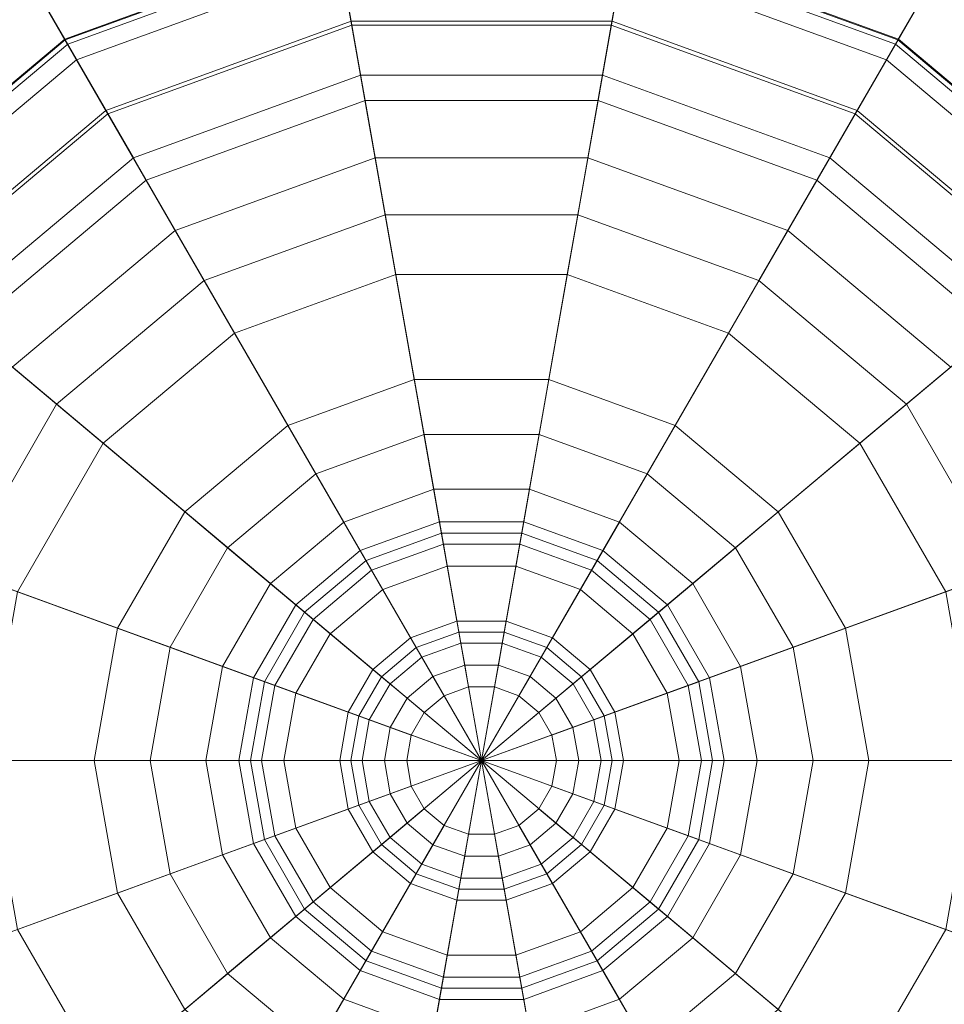
# Model space of a CAD drawing. Units: inches. Extents: x 375 to 1122, y 27 to 1069.
# Tile 141 of 155: x 732.384 to 733.741, y 898.759 to 900.205. Entities that reach past the tile are written whole.
import ezdxf

# ---------------------------------------------------------------- set-up
doc = ezdxf.new("R2010")
doc.units = ezdxf.units.IN
doc.layers.add('A-ANNO-DIMS', color=2, linetype='Continuous', lineweight=18)
doc.layers.add('Furniture', color=30, linetype='Continuous', lineweight=18)
doc.styles.get("Standard").update_dxf_attribs({"font": 'arial.ttf'})
doc.dimstyles.new('ISO-25', dxfattribs={"dimtxt": 12, "dimasz": 2.5, "dimexe": 1.5, "dimexo": 1.5, "dimtad": 1, "dimdec": 1, "dimlunit": 3, "dimtxsty": 'Standard', "dimblk": 'ARCHTICK', "dimcen": 2.5, "dimadec": 0, "dimazin": 0, "dimtfac": 1, "dimtdec": 1, "dimtmove": 0, "dimatfit": 3, "dimfxl": 1.5, "dimfxlon": 1, "dimarcsym": 0})

# ---------------------------------------------------------------- blocks, each defined once
blk = doc.blocks.new('A$C403C54AD')
for points in [[(0.980157, 1.23678, -0.04658), (0.980157, 1.202917, -0.043501), (0.980157, 1.202917, -0.043501), (0.968576, 1.234737, -0.04658)], [(0.991739, 1.234737, -0.04658), (0.980157, 1.202917, -0.043501), (0.980157, 1.202917, -0.043501), (0.980157, 1.23678, -0.04658)], [(0.968576, 1.234737, -0.04658), (0.980157, 1.202917, -0.043501), (0.980157, 1.202917, -0.043501), (0.958391, 1.228857, -0.04658)], [(1.001923, 1.228857, -0.04658), (0.980157, 1.202917, -0.043501), (0.980157, 1.202917, -0.043501), (0.991739, 1.234737, -0.04658)], [(0.980157, 1.217132, -0.040074), (0.980157, 1.233514, -0.043349), (0.969693, 1.231669, -0.043349), (0.975296, 1.216274, -0.040074)], [(0.985019, 1.216274, -0.040074), (0.990622, 1.231669, -0.043349), (0.980157, 1.233514, -0.043349), (0.980157, 1.217132, -0.040074)], [(0.975296, 1.216274, -0.040074), (0.969693, 1.231669, -0.043349), (0.96049, 1.226356, -0.043349), (0.971021, 1.213806, -0.040074)], [(0.989294, 1.213806, -0.040074), (0.999824, 1.226356, -0.043349), (0.990622, 1.231669, -0.043349), (0.985019, 1.216274, -0.040074)], [(0.958391, 1.228857, -0.04658), (0.980157, 1.202917, -0.043501), (0.980157, 1.202917, -0.043501), (0.950832, 1.219849, -0.04658)], [(0.96049, 1.226356, -0.043349), (0.958391, 1.228857, -0.04658), (0.950832, 1.219849, -0.04658), (0.95366, 1.218216, -0.043349)], [(0.960516, 1.226325, 0.116404), (0.958647, 1.228552, 0.10318), (0.951177, 1.219649, 0.10318), (0.953695, 1.218195, 0.116404)], [(0.958647, 1.228552, 0.10318), (0.959081, 1.228035, 0.074938), (0.951762, 1.219312, 0.074938), (0.951177, 1.219649, 0.10318)], [(0.970778, 1.228687, 0.056929), (0.973195, 1.222047, 0.046697), (0.967072, 1.218512, 0.046697), (0.96253, 1.223925, 0.056929)], [(1.009483, 1.219849, -0.04658), (0.980157, 1.202917, -0.043501), (0.980157, 1.202917, -0.043501), (1.001923, 1.228857, -0.04658)], [(0.997785, 1.223925, 0.056929), (0.993243, 1.218512, 0.046697), (0.98712, 1.222047, 0.046697), (0.989537, 1.228687, 0.056929)], [(0.959081, 1.228035, 0.074938), (0.96253, 1.223925, 0.056929), (0.956408, 1.216629, 0.056929), (0.951762, 1.219312, 0.074938)], [(0.971021, 1.213806, -0.040074), (0.96049, 1.226356, -0.043349), (0.95366, 1.218216, -0.043349), (0.967847, 1.210025, -0.040074)], [(0.963728, 1.222497, 0.12581), (0.960516, 1.226325, 0.116404), (0.953695, 1.218195, 0.116404), (0.958022, 1.215697, 0.12581)], [(0.96063, 1.226189, 0.102963), (0.962436, 1.224037, 0.115599), (0.956282, 1.216702, 0.115599), (0.953848, 1.218107, 0.102963)], [(0.961053, 1.225685, 0.075423), (0.96063, 1.226189, 0.102963), (0.953848, 1.218107, 0.102963), (0.954418, 1.217778, 0.075423)], [(0.973957, 1.219951, 0.048884), (0.971739, 1.226046, 0.058276), (0.964336, 1.221772, 0.058276), (0.968505, 1.216804, 0.048884)], [(0.991809, 1.216804, 0.048884), (0.995978, 1.221772, 0.058276), (0.988575, 1.226046, 0.058276), (0.986357, 1.219951, 0.048884)], [(0.964336, 1.221772, 0.058276), (0.961053, 1.225685, 0.075423), (0.954418, 1.217778, 0.075423), (0.958842, 1.215224, 0.058276)], [(0.962436, 1.224037, 0.115599), (0.965707, 1.220139, 0.12581), (0.960688, 1.214158, 0.12581), (0.956282, 1.216702, 0.115599)], [(0.96253, 1.223925, 0.056929), (0.967072, 1.218512, 0.046697), (0.962527, 1.213096, 0.046697), (0.956408, 1.216629, 0.056929)], [(0.980157, 1.223275, 0.046697), (0.980157, 1.213036, 0.03933), (0.976696, 1.212426, 0.03933), (0.973195, 1.222047, 0.046697)], [(0.98712, 1.222047, 0.046697), (0.983618, 1.212426, 0.03933), (0.980157, 1.213036, 0.03933), (0.980157, 1.223275, 0.046697)], [(0.965707, 1.220139, 0.12581), (0.963728, 1.222497, 0.12581), (0.958022, 1.215697, 0.12581), (0.960688, 1.214158, 0.12581)], [(0.973195, 1.222047, 0.046697), (0.976696, 1.212426, 0.03933), (0.973653, 1.210669, 0.03933), (0.967072, 1.218512, 0.046697)], [(0.993243, 1.218512, 0.046697), (0.986661, 1.210669, 0.03933), (0.983618, 1.212426, 0.03933), (0.98712, 1.222047, 0.046697)], [(0.968505, 1.216804, 0.048884), (0.964336, 1.221772, 0.058276), (0.958842, 1.215224, 0.058276), (0.964459, 1.211981, 0.048884)], [(0.980157, 1.211822, 0.042248), (0.980157, 1.221045, 0.048884), (0.973957, 1.219951, 0.048884), (0.977112, 1.211285, 0.042248)], [(0.983203, 1.211285, 0.042248), (0.986357, 1.219951, 0.048884), (0.980157, 1.221045, 0.048884), (0.980157, 1.211822, 0.042248)], [(0.977112, 1.211285, 0.042248), (0.973957, 1.219951, 0.048884), (0.968505, 1.216804, 0.048884), (0.974434, 1.209738, 0.042248)], [(0.985881, 1.209738, 0.042248), (0.991809, 1.216804, 0.048884), (0.986357, 1.219951, 0.048884), (0.983203, 1.211285, 0.042248)], [(0.950832, 1.219849, -0.04658), (0.980157, 1.202917, -0.043501), (0.980157, 1.202917, -0.043501), (0.94681, 1.208798, -0.04658)], [(0.95366, 1.218216, -0.043349), (0.950832, 1.219849, -0.04658), (0.94681, 1.208798, -0.04658), (0.950026, 1.20823, -0.043349)], [(0.953695, 1.218195, 0.116404), (0.951177, 1.219649, 0.10318), (0.947202, 1.208728, 0.10318), (0.950065, 1.208223, 0.116404)], [(1.013505, 1.208798, -0.04658), (0.980157, 1.202917, -0.043501), (0.980157, 1.202917, -0.043501), (1.009483, 1.219849, -0.04658)], [(0.951762, 1.219312, 0.074938), (0.956408, 1.216629, 0.056929), (0.95315, 1.20768, 0.056929), (0.947867, 1.208611, 0.074938)], [(0.967072, 1.218512, 0.046697), (0.973653, 1.210669, 0.03933), (0.971394, 1.207977, 0.03933), (0.962527, 1.213096, 0.046697)], [(0.997787, 1.213096, 0.046697), (0.98892, 1.207977, 0.03933), (0.986661, 1.210669, 0.03933), (0.993243, 1.218512, 0.046697)], [(0.967847, 1.210025, -0.040074), (0.95366, 1.218216, -0.043349), (0.950026, 1.20823, -0.043349), (0.966159, 1.205386, -0.040074)], [(0.958022, 1.215697, 0.12581), (0.953695, 1.218195, 0.116404), (0.950065, 1.208223, 0.116404), (0.954986, 1.207356, 0.12581)], [(0.953848, 1.218107, 0.102963), (0.956282, 1.216702, 0.115599), (0.953007, 1.207705, 0.115599), (0.95024, 1.208193, 0.102963)], [(0.954418, 1.217778, 0.075423), (0.953848, 1.218107, 0.102963), (0.95024, 1.208193, 0.102963), (0.950888, 1.208078, 0.075423)], [(0.958842, 1.215224, 0.058276), (0.954418, 1.217778, 0.075423), (0.950888, 1.208078, 0.075423), (0.955918, 1.207191, 0.058276)], [(0.980157, 1.215084, -0.037209), (0.980157, 1.217132, -0.040074), (0.975296, 1.216274, -0.040074), (0.975996, 1.21435, -0.037209)], [(0.984318, 1.21435, -0.037209), (0.985019, 1.216274, -0.040074), (0.980157, 1.217132, -0.040074), (0.980157, 1.215084, -0.037209)], [(0.956282, 1.216702, 0.115599), (0.960688, 1.214158, 0.12581), (0.958018, 1.206821, 0.12581), (0.953007, 1.207705, 0.115599)], [(0.956408, 1.216629, 0.056929), (0.962527, 1.213096, 0.046697), (0.960109, 1.206452, 0.046697), (0.95315, 1.20768, 0.056929)], [(0.974434, 1.209738, 0.042248), (0.968505, 1.216804, 0.048884), (0.964459, 1.211981, 0.048884), (0.972446, 1.207369, 0.042248)], [(0.987868, 1.207369, 0.042248), (0.995856, 1.211981, 0.048884), (0.991809, 1.216804, 0.048884), (0.985881, 1.209738, 0.042248)], [(0.975996, 1.21435, -0.037209), (0.975296, 1.216274, -0.040074), (0.971021, 1.213806, -0.040074), (0.972337, 1.212238, -0.037209)], [(0.987978, 1.212238, -0.037209), (0.989294, 1.213806, -0.040074), (0.985019, 1.216274, -0.040074), (0.984318, 1.21435, -0.037209)], [(0.960688, 1.214158, 0.12581), (0.958022, 1.215697, 0.12581), (0.954986, 1.207356, 0.12581), (0.958018, 1.206821, 0.12581)], [(0.964459, 1.211981, 0.048884), (0.958842, 1.215224, 0.058276), (0.955918, 1.207191, 0.058276), (0.962305, 1.206065, 0.048884)], [(0.980157, 1.210988, -0.035163), (0.980157, 1.215084, -0.037209), (0.975996, 1.21435, -0.037209), (0.977397, 1.210502, -0.035163)], [(0.982918, 1.210502, -0.035163), (0.984318, 1.21435, -0.037209), (0.980157, 1.215084, -0.037209), (0.980157, 1.210988, -0.035163)], [(0.977397, 1.210502, -0.035163), (0.975996, 1.21435, -0.037209), (0.972337, 1.212238, -0.037209), (0.974969, 1.2091, -0.035163)], [(0.985345, 1.2091, -0.035163), (0.987978, 1.212238, -0.037209), (0.984318, 1.21435, -0.037209), (0.982918, 1.210502, -0.035163)], [(0.972337, 1.212238, -0.037209), (0.971021, 1.213806, -0.040074), (0.967847, 1.210025, -0.040074), (0.969621, 1.209001, -0.037209)], [(0.990694, 1.209001, -0.037209), (0.992467, 1.210025, -0.040074), (0.989294, 1.213806, -0.040074), (0.987978, 1.212238, -0.037209)], [(0.962527, 1.213096, 0.046697), (0.971394, 1.207977, 0.03933), (0.970192, 1.204675, 0.03933), (0.960109, 1.206452, 0.046697)], [(0.980157, 1.213036, 0.03933), (0.980157, 1.208122, 0.038511), (0.978377, 1.207808, 0.038511), (0.976696, 1.212426, 0.03933)], [(0.983618, 1.212426, 0.03933), (0.981937, 1.207808, 0.038511), (0.980157, 1.208122, 0.038511), (0.980157, 1.213036, 0.03933)], [(1.000206, 1.206452, 0.046697), (0.990122, 1.204675, 0.03933), (0.98892, 1.207977, 0.03933), (0.997787, 1.213096, 0.046697)], [(0.976696, 1.212426, 0.03933), (0.978377, 1.207808, 0.038511), (0.976812, 1.206904, 0.038511), (0.973653, 1.210669, 0.03933)], [(0.986661, 1.210669, 0.03933), (0.983502, 1.206904, 0.038511), (0.981937, 1.207808, 0.038511), (0.983618, 1.212426, 0.03933)], [(0.972446, 1.207369, 0.042248), (0.964459, 1.211981, 0.048884), (0.962305, 1.206065, 0.048884), (0.971388, 1.204464, 0.042248)], [(0.974969, 1.2091, -0.035163), (0.972337, 1.212238, -0.037209), (0.969621, 1.209001, -0.037209), (0.973168, 1.206953, -0.035163)], [(0.987147, 1.206953, -0.035163), (0.990694, 1.209001, -0.037209), (0.987978, 1.212238, -0.037209), (0.985345, 1.2091, -0.035163)], [(0.988926, 1.204464, 0.042248), (0.998009, 1.206065, 0.048884), (0.995856, 1.211981, 0.048884), (0.987868, 1.207369, 0.042248)], [(0.980157, 1.202917, 0.040765), (0.980157, 1.211822, 0.042248), (0.977112, 1.211285, 0.042248), (0.980157, 1.202917, 0.040765)], [(0.980157, 1.202917, 0.040765), (0.983203, 1.211285, 0.042248), (0.980157, 1.211822, 0.042248), (0.980157, 1.202917, 0.040765)], [(0.980157, 1.202917, 0.040765), (0.977112, 1.211285, 0.042248), (0.974434, 1.209738, 0.042248), (0.980157, 1.202917, 0.040765)], [(0.980157, 1.211398, 0.035646), (0.980157, 1.207302, 0.033599), (0.978658, 1.207038, 0.033599), (0.977257, 1.210887, 0.035646)], [(0.980157, 1.210169, 0.037692), (0.980157, 1.211398, 0.035646), (0.977257, 1.210887, 0.035646), (0.977677, 1.209732, 0.037692)], [(0.983058, 1.210887, 0.035646), (0.981657, 1.207038, 0.033599), (0.980157, 1.207302, 0.033599), (0.980157, 1.211398, 0.035646)], [(0.982638, 1.209732, 0.037692), (0.983058, 1.210887, 0.035646), (0.980157, 1.211398, 0.035646), (0.980157, 1.210169, 0.037692)], [(0.980157, 1.202917, 0.040765), (0.985881, 1.209738, 0.042248), (0.983203, 1.211285, 0.042248), (0.980157, 1.202917, 0.040765)], [(0.977257, 1.210887, 0.035646), (0.978658, 1.207038, 0.033599), (0.977339, 1.206277, 0.033599), (0.974706, 1.209414, 0.035646)], [(0.977677, 1.209732, 0.037692), (0.977257, 1.210887, 0.035646), (0.974706, 1.209414, 0.035646), (0.975496, 1.208473, 0.037692)], [(0.980157, 1.207712, -0.029842), (0.980157, 1.210988, -0.035163), (0.977397, 1.210502, -0.035163), (0.978517, 1.207423, -0.029842)], [(0.981797, 1.207423, -0.029842), (0.982918, 1.210502, -0.035163), (0.980157, 1.210988, -0.035163), (0.980157, 1.207712, -0.029842)], [(0.985608, 1.209414, 0.035646), (0.982976, 1.206277, 0.033599), (0.981657, 1.207038, 0.033599), (0.983058, 1.210887, 0.035646)], [(0.984819, 1.208473, 0.037692), (0.985608, 1.209414, 0.035646), (0.983058, 1.210887, 0.035646), (0.982638, 1.209732, 0.037692)], [(0.973653, 1.210669, 0.03933), (0.976812, 1.206904, 0.038511), (0.97565, 1.205519, 0.038511), (0.971394, 1.207977, 0.03933)], [(0.978517, 1.207423, -0.029842), (0.977397, 1.210502, -0.035163), (0.974969, 1.2091, -0.035163), (0.977075, 1.20659, -0.029842)], [(0.983239, 1.20659, -0.029842), (0.985345, 1.2091, -0.035163), (0.982918, 1.210502, -0.035163), (0.981797, 1.207423, -0.029842)], [(0.98892, 1.207977, 0.03933), (0.984664, 1.205519, 0.038511), (0.983502, 1.206904, 0.038511), (0.986661, 1.210669, 0.03933)], [(0.980157, 1.208122, 0.038511), (0.980157, 1.210169, 0.037692), (0.977677, 1.209732, 0.037692), (0.978377, 1.207808, 0.038511)], [(0.981937, 1.207808, 0.038511), (0.982638, 1.209732, 0.037692), (0.980157, 1.210169, 0.037692), (0.980157, 1.208122, 0.038511)], [(0.969621, 1.209001, -0.037209), (0.967847, 1.210025, -0.040074), (0.966159, 1.205386, -0.040074), (0.968176, 1.20503, -0.037209)], [(0.980157, 1.202917, 0.040765), (0.974434, 1.209738, 0.042248), (0.972446, 1.207369, 0.042248), (0.980157, 1.202917, 0.040765)], [(0.980157, 1.202917, 0.040765), (0.987868, 1.207369, 0.042248), (0.985881, 1.209738, 0.042248), (0.980157, 1.202917, 0.040765)], [(0.974706, 1.209414, 0.035646), (0.977339, 1.206277, 0.033599), (0.97636, 1.20511, 0.033599), (0.972813, 1.207158, 0.035646)], [(0.975496, 1.208473, 0.037692), (0.974706, 1.209414, 0.035646), (0.972813, 1.207158, 0.035646), (0.973877, 1.206543, 0.037692)], [(0.978377, 1.207808, 0.038511), (0.977677, 1.209732, 0.037692), (0.975496, 1.208473, 0.037692), (0.976812, 1.206904, 0.038511)], [(0.983502, 1.206904, 0.038511), (0.984819, 1.208473, 0.037692), (0.982638, 1.209732, 0.037692), (0.981937, 1.207808, 0.038511)], [(0.987502, 1.207158, 0.035646), (0.983955, 1.20511, 0.033599), (0.982976, 1.206277, 0.033599), (0.985608, 1.209414, 0.035646)], [(0.986438, 1.206543, 0.037692), (0.987502, 1.207158, 0.035646), (0.985608, 1.209414, 0.035646), (0.984819, 1.208473, 0.037692)], [(0.977075, 1.20659, -0.029842), (0.974969, 1.2091, -0.035163), (0.973168, 1.206953, -0.035163), (0.976005, 1.205315, -0.029842)], [(0.98431, 1.205315, -0.029842), (0.987147, 1.206953, -0.035163), (0.985345, 1.2091, -0.035163), (0.983239, 1.20659, -0.029842)], [(0.94681, 1.208798, -0.04658), (0.980157, 1.202917, -0.043501), (0.980157, 1.202917, -0.043501), (0.94681, 1.197037, -0.04658)], [(0.973168, 1.206953, -0.035163), (0.969621, 1.209001, -0.037209), (0.968176, 1.20503, -0.037209), (0.972209, 1.204319, -0.035163)], [(1.013505, 1.197037, -0.04658), (0.980157, 1.202917, -0.043501), (0.980157, 1.202917, -0.043501), (1.013505, 1.208798, -0.04658)], [(0.988106, 1.204319, -0.035163), (0.992139, 1.20503, -0.037209), (0.990694, 1.209001, -0.037209), (0.987147, 1.206953, -0.035163)], [(0.947867, 1.208611, 0.074938), (0.95315, 1.20768, 0.056929), (0.95315, 1.198155, 0.056929), (0.947867, 1.197224, 0.074938)], [(0.976812, 1.206904, 0.038511), (0.975496, 1.208473, 0.037692), (0.973877, 1.206543, 0.037692), (0.97565, 1.205519, 0.038511)], [(0.984664, 1.205519, 0.038511), (0.986438, 1.206543, 0.037692), (0.984819, 1.208473, 0.037692), (0.983502, 1.206904, 0.038511)], [(0.966159, 1.205386, -0.040074), (0.950026, 1.20823, -0.043349), (0.950026, 1.197604, -0.043349), (0.966159, 1.200449, -0.040074)], [(0.954986, 1.207356, 0.12581), (0.950065, 1.208223, 0.116404), (0.950065, 1.197611, 0.116404), (0.954986, 1.198479, 0.12581)], [(0.95024, 1.208193, 0.102963), (0.953007, 1.207705, 0.115599), (0.953007, 1.19813, 0.115599), (0.95024, 1.197642, 0.102963)], [(0.955918, 1.207191, 0.058276), (0.950888, 1.208078, 0.075423), (0.950888, 1.197756, 0.075423), (0.955918, 1.198643, 0.058276)], [(0.971394, 1.207977, 0.03933), (0.97565, 1.205519, 0.038511), (0.975032, 1.203821, 0.038511), (0.970192, 1.204675, 0.03933)], [(0.990122, 1.204675, 0.03933), (0.985282, 1.203821, 0.038511), (0.984664, 1.205519, 0.038511), (0.98892, 1.207977, 0.03933)], [(0.953007, 1.207705, 0.115599), (0.958018, 1.206821, 0.12581), (0.958018, 1.199014, 0.12581), (0.953007, 1.19813, 0.115599)], [(0.95315, 1.20768, 0.056929), (0.960109, 1.206452, 0.046697), (0.960109, 1.199382, 0.046697), (0.95315, 1.198155, 0.056929)], [(0.980157, 1.206483, -0.021247), (0.980157, 1.207712, -0.029842), (0.978517, 1.207423, -0.029842), (0.978938, 1.206268, -0.021247)], [(0.981377, 1.206268, -0.021247), (0.981797, 1.207423, -0.029842), (0.980157, 1.207712, -0.029842), (0.980157, 1.206483, -0.021247)], [(0.958018, 1.206821, 0.12581), (0.954986, 1.207356, 0.12581), (0.954986, 1.198479, 0.12581), (0.958018, 1.199014, 0.12581)], [(0.980157, 1.202917, 0.040765), (0.972446, 1.207369, 0.042248), (0.971388, 1.204464, 0.042248), (0.980157, 1.202917, 0.040765)], [(0.978938, 1.206268, -0.021247), (0.978517, 1.207423, -0.029842), (0.977075, 1.20659, -0.029842), (0.977865, 1.205649, -0.021247)], [(0.980157, 1.207302, 0.033599), (0.980157, 1.205664, 0.027051), (0.979218, 1.205499, 0.027051), (0.978658, 1.207038, 0.033599)], [(0.980157, 1.202917, 0.040765), (0.988926, 1.204464, 0.042248), (0.987868, 1.207369, 0.042248), (0.980157, 1.202917, 0.040765)], [(0.981657, 1.207038, 0.033599), (0.981097, 1.205499, 0.027051), (0.980157, 1.205664, 0.027051), (0.980157, 1.207302, 0.033599)], [(0.982449, 1.205649, -0.021247), (0.983239, 1.20659, -0.029842), (0.981797, 1.207423, -0.029842), (0.981377, 1.206268, -0.021247)], [(0.962305, 1.206065, 0.048884), (0.955918, 1.207191, 0.058276), (0.955918, 1.198643, 0.058276), (0.962305, 1.19977, 0.048884)], [(0.972813, 1.207158, 0.035646), (0.97636, 1.20511, 0.033599), (0.975839, 1.203679, 0.033599), (0.971806, 1.20439, 0.035646)], [(0.973877, 1.206543, 0.037692), (0.972813, 1.207158, 0.035646), (0.971806, 1.20439, 0.035646), (0.973016, 1.204177, 0.037692)], [(0.976005, 1.205315, -0.029842), (0.973168, 1.206953, -0.035163), (0.972209, 1.204319, -0.035163), (0.975436, 1.20375, -0.029842)], [(0.978658, 1.207038, 0.033599), (0.979218, 1.205499, 0.027051), (0.978392, 1.205022, 0.027051), (0.977339, 1.206277, 0.033599)], [(0.982976, 1.206277, 0.033599), (0.981923, 1.205022, 0.027051), (0.981097, 1.205499, 0.027051), (0.981657, 1.207038, 0.033599)], [(0.988509, 1.20439, 0.035646), (0.984476, 1.203679, 0.033599), (0.983955, 1.20511, 0.033599), (0.987502, 1.207158, 0.035646)], [(0.984879, 1.20375, -0.029842), (0.988106, 1.204319, -0.035163), (0.987147, 1.206953, -0.035163), (0.98431, 1.205315, -0.029842)], [(0.987299, 1.204177, 0.037692), (0.988509, 1.20439, 0.035646), (0.987502, 1.207158, 0.035646), (0.986438, 1.206543, 0.037692)], [(0.97565, 1.205519, 0.038511), (0.973877, 1.206543, 0.037692), (0.973016, 1.204177, 0.037692), (0.975032, 1.203821, 0.038511)], [(0.977865, 1.205649, -0.021247), (0.977075, 1.20659, -0.029842), (0.976005, 1.205315, -0.029842), (0.977069, 1.2047, -0.021247)], [(0.983245, 1.2047, -0.021247), (0.98431, 1.205315, -0.029842), (0.983239, 1.20659, -0.029842), (0.982449, 1.205649, -0.021247)], [(0.985282, 1.203821, 0.038511), (0.987299, 1.204177, 0.037692), (0.986438, 1.206543, 0.037692), (0.984664, 1.205519, 0.038511)], [(0.960109, 1.206452, 0.046697), (0.970192, 1.204675, 0.03933), (0.970192, 1.20116, 0.03933), (0.960109, 1.199382, 0.046697)], [(0.977339, 1.206277, 0.033599), (0.978392, 1.205022, 0.027051), (0.977778, 1.204291, 0.027051), (0.97636, 1.20511, 0.033599)], [(0.979218, 1.205499, 0.027051), (0.978938, 1.206268, -0.021247), (0.977865, 1.205649, -0.021247), (0.978392, 1.205022, 0.027051)], [(0.980157, 1.205664, 0.027051), (0.980157, 1.206483, -0.021247), (0.978938, 1.206268, -0.021247), (0.979218, 1.205499, 0.027051)], [(0.981097, 1.205499, 0.027051), (0.981377, 1.206268, -0.021247), (0.980157, 1.206483, -0.021247), (0.980157, 1.205664, 0.027051)], [(0.981923, 1.205022, 0.027051), (0.982449, 1.205649, -0.021247), (0.981377, 1.206268, -0.021247), (0.981097, 1.205499, 0.027051)], [(0.983955, 1.20511, 0.033599), (0.982536, 1.204291, 0.027051), (0.981923, 1.205022, 0.027051), (0.982976, 1.206277, 0.033599)], [(0.971388, 1.204464, 0.042248), (0.962305, 1.206065, 0.048884), (0.962305, 1.19977, 0.048884), (0.971388, 1.201371, 0.042248)], [(0.988926, 1.201371, 0.042248), (0.998009, 1.19977, 0.048884), (0.998009, 1.206065, 0.048884), (0.988926, 1.204464, 0.042248)], [(0.978392, 1.205022, 0.027051), (0.977865, 1.205649, -0.021247), (0.977069, 1.2047, -0.021247), (0.977778, 1.204291, 0.027051)], [(0.982536, 1.204291, 0.027051), (0.983245, 1.2047, -0.021247), (0.982449, 1.205649, -0.021247), (0.981923, 1.205022, 0.027051)], [(0.968176, 1.20503, -0.037209), (0.966159, 1.205386, -0.040074), (0.966159, 1.200449, -0.040074), (0.968176, 1.200805, -0.037209)], [(0.977069, 1.2047, -0.021247), (0.976005, 1.205315, -0.029842), (0.975436, 1.20375, -0.029842), (0.976646, 1.203537, -0.021247)], [(0.97636, 1.20511, 0.033599), (0.977778, 1.204291, 0.027051), (0.977452, 1.203394, 0.027051), (0.975839, 1.203679, 0.033599)], [(0.984476, 1.203679, 0.033599), (0.982862, 1.203394, 0.027051), (0.982536, 1.204291, 0.027051), (0.983955, 1.20511, 0.033599)], [(0.983669, 1.203537, -0.021247), (0.984879, 1.20375, -0.029842), (0.98431, 1.205315, -0.029842), (0.983245, 1.2047, -0.021247)], [(0.972209, 1.204319, -0.035163), (0.968176, 1.20503, -0.037209), (0.968176, 1.200805, -0.037209), (0.972209, 1.201516, -0.035163)], [(0.977778, 1.204291, 0.027051), (0.977069, 1.2047, -0.021247), (0.976646, 1.203537, -0.021247), (0.977452, 1.203394, 0.027051)], [(0.982862, 1.203394, 0.027051), (0.983669, 1.203537, -0.021247), (0.983245, 1.2047, -0.021247), (0.982536, 1.204291, 0.027051)], [(0.988106, 1.201516, -0.035163), (0.992139, 1.200805, -0.037209), (0.992139, 1.20503, -0.037209), (0.988106, 1.204319, -0.035163)], [(0.970192, 1.204675, 0.03933), (0.975032, 1.203821, 0.038511), (0.975032, 1.202014, 0.038511), (0.970192, 1.20116, 0.03933)], [(0.980157, 1.202917, 0.040765), (0.971388, 1.204464, 0.042248), (0.971388, 1.201371, 0.042248), (0.980157, 1.202917, 0.040765)], [(0.971806, 1.20439, 0.035646), (0.975839, 1.203679, 0.033599), (0.975839, 1.202156, 0.033599), (0.971806, 1.201445, 0.035646)], [(0.973016, 1.204177, 0.037692), (0.971806, 1.20439, 0.035646), (0.971806, 1.201445, 0.035646), (0.973016, 1.201658, 0.037692)], [(0.975436, 1.20375, -0.029842), (0.972209, 1.204319, -0.035163), (0.972209, 1.201516, -0.035163), (0.975436, 1.202085, -0.029842)], [(0.980157, 1.202917, 0.040765), (0.988926, 1.201371, 0.042248), (0.988926, 1.204464, 0.042248), (0.980157, 1.202917, 0.040765)], [(0.988509, 1.201445, 0.035646), (0.984476, 1.202156, 0.033599), (0.984476, 1.203679, 0.033599), (0.988509, 1.20439, 0.035646)], [(0.984879, 1.202085, -0.029842), (0.988106, 1.201516, -0.035163), (0.988106, 1.204319, -0.035163), (0.984879, 1.20375, -0.029842)], [(0.990122, 1.20116, 0.03933), (0.985282, 1.202014, 0.038511), (0.985282, 1.203821, 0.038511), (0.990122, 1.204675, 0.03933)], [(0.987299, 1.201658, 0.037692), (0.988509, 1.201445, 0.035646), (0.988509, 1.20439, 0.035646), (0.987299, 1.204177, 0.037692)], [(0.975032, 1.203821, 0.038511), (0.973016, 1.204177, 0.037692), (0.973016, 1.201658, 0.037692), (0.975032, 1.202014, 0.038511)], [(0.985282, 1.202014, 0.038511), (0.987299, 1.201658, 0.037692), (0.987299, 1.204177, 0.037692), (0.985282, 1.203821, 0.038511)], [(0.976646, 1.203537, -0.021247), (0.975436, 1.20375, -0.029842), (0.975436, 1.202085, -0.029842), (0.976646, 1.202298, -0.021247)], [(0.975839, 1.203679, 0.033599), (0.977452, 1.203394, 0.027051), (0.977452, 1.20244, 0.027051), (0.975839, 1.202156, 0.033599)], [(0.984476, 1.202156, 0.033599), (0.982862, 1.20244, 0.027051), (0.982862, 1.203394, 0.027051), (0.984476, 1.203679, 0.033599)], [(0.983669, 1.202298, -0.021247), (0.984879, 1.202085, -0.029842), (0.984879, 1.20375, -0.029842), (0.983669, 1.203537, -0.021247)], [(0.977452, 1.203394, 0.027051), (0.976646, 1.203537, -0.021247), (0.976646, 1.202298, -0.021247), (0.977452, 1.20244, 0.027051)], [(0.982862, 1.20244, 0.027051), (0.983669, 1.202298, -0.021247), (0.983669, 1.203537, -0.021247), (0.982862, 1.203394, 0.027051)], [(0.94681, 1.197037, -0.04658), (0.980157, 1.202917, -0.043501), (0.980157, 1.202917, -0.043501), (0.950832, 1.185986, -0.04658)], [(0.950832, 1.185986, -0.04658), (0.980157, 1.202917, -0.043501), (0.980157, 1.202917, -0.043501), (0.958391, 1.176977, -0.04658)], [(0.958391, 1.176977, -0.04658), (0.980157, 1.202917, -0.043501), (0.980157, 1.202917, -0.043501), (0.968576, 1.171097, -0.04658)], [(0.968576, 1.171097, -0.04658), (0.980157, 1.202917, -0.043501), (0.980157, 1.202917, -0.043501), (0.980157, 1.169055, -0.04658)], [(0.980157, 1.202917, 0.040765), (0.971388, 1.201371, 0.042248), (0.972446, 1.198465, 0.042248), (0.980157, 1.202917, 0.040765)], [(0.980157, 1.202917, 0.040765), (0.972446, 1.198465, 0.042248), (0.974434, 1.196096, 0.042248), (0.980157, 1.202917, 0.040765)], [(0.980157, 1.202917, 0.040765), (0.974434, 1.196096, 0.042248), (0.977112, 1.19455, 0.042248), (0.980157, 1.202917, 0.040765)], [(0.980157, 1.202917, 0.040765), (0.977112, 1.19455, 0.042248), (0.980157, 1.194013, 0.042248), (0.980157, 1.202917, 0.040765)], [(0.980157, 1.202917, 0.040765), (0.983203, 1.19455, 0.042248), (0.985881, 1.196096, 0.042248), (0.980157, 1.202917, 0.040765)], [(0.980157, 1.202917, 0.040765), (0.980157, 1.194013, 0.042248), (0.983203, 1.19455, 0.042248), (0.980157, 1.202917, 0.040765)], [(0.980157, 1.202917, 0.040765), (0.987868, 1.198465, 0.042248), (0.988926, 1.201371, 0.042248), (0.980157, 1.202917, 0.040765)], [(0.980157, 1.202917, 0.040765), (0.985881, 1.196096, 0.042248), (0.987868, 1.198465, 0.042248), (0.980157, 1.202917, 0.040765)], [(1.009483, 1.185986, -0.04658), (0.980157, 1.202917, -0.043501), (0.980157, 1.202917, -0.043501), (1.013505, 1.197037, -0.04658)], [(1.001923, 1.176977, -0.04658), (0.980157, 1.202917, -0.043501), (0.980157, 1.202917, -0.043501), (1.009483, 1.185986, -0.04658)], [(0.991739, 1.171097, -0.04658), (0.980157, 1.202917, -0.043501), (0.980157, 1.202917, -0.043501), (1.001923, 1.176977, -0.04658)], [(0.980157, 1.169055, -0.04658), (0.980157, 1.202917, -0.043501), (0.980157, 1.202917, -0.043501), (0.991739, 1.171097, -0.04658)], [(0.971806, 1.201445, 0.035646), (0.975839, 1.202156, 0.033599), (0.97636, 1.200725, 0.033599), (0.972813, 1.198677, 0.035646)], [(0.976646, 1.202298, -0.021247), (0.975436, 1.202085, -0.029842), (0.976005, 1.20052, -0.029842), (0.977069, 1.201134, -0.021247)], [(0.975839, 1.202156, 0.033599), (0.977452, 1.20244, 0.027051), (0.977778, 1.201544, 0.027051), (0.97636, 1.200725, 0.033599)], [(0.977452, 1.20244, 0.027051), (0.976646, 1.202298, -0.021247), (0.977069, 1.201134, -0.021247), (0.977778, 1.201544, 0.027051)], [(0.983955, 1.200725, 0.033599), (0.982536, 1.201544, 0.027051), (0.982862, 1.20244, 0.027051), (0.984476, 1.202156, 0.033599)], [(0.982536, 1.201544, 0.027051), (0.983245, 1.201134, -0.021247), (0.983669, 1.202298, -0.021247), (0.982862, 1.20244, 0.027051)], [(0.983245, 1.201134, -0.021247), (0.98431, 1.20052, -0.029842), (0.984879, 1.202085, -0.029842), (0.983669, 1.202298, -0.021247)], [(0.987502, 1.198677, 0.035646), (0.983955, 1.200725, 0.033599), (0.984476, 1.202156, 0.033599), (0.988509, 1.201445, 0.035646)], [(0.970192, 1.20116, 0.03933), (0.975032, 1.202014, 0.038511), (0.97565, 1.200315, 0.038511), (0.971394, 1.197858, 0.03933)], [(0.975436, 1.202085, -0.029842), (0.972209, 1.201516, -0.035163), (0.973168, 1.198882, -0.035163), (0.976005, 1.20052, -0.029842)], [(0.975032, 1.202014, 0.038511), (0.973016, 1.201658, 0.037692), (0.973877, 1.199291, 0.037692), (0.97565, 1.200315, 0.038511)], [(0.98431, 1.20052, -0.029842), (0.987147, 1.198882, -0.035163), (0.988106, 1.201516, -0.035163), (0.984879, 1.202085, -0.029842)], [(0.984664, 1.200315, 0.038511), (0.986438, 1.199291, 0.037692), (0.987299, 1.201658, 0.037692), (0.985282, 1.202014, 0.038511)], [(0.98892, 1.197858, 0.03933), (0.984664, 1.200315, 0.038511), (0.985282, 1.202014, 0.038511), (0.990122, 1.20116, 0.03933)], [(0.972209, 1.201516, -0.035163), (0.968176, 1.200805, -0.037209), (0.969621, 1.196834, -0.037209), (0.973168, 1.198882, -0.035163)], [(0.973016, 1.201658, 0.037692), (0.971806, 1.201445, 0.035646), (0.972813, 1.198677, 0.035646), (0.973877, 1.199291, 0.037692)], [(0.97636, 1.200725, 0.033599), (0.977778, 1.201544, 0.027051), (0.978392, 1.200813, 0.027051), (0.977339, 1.199558, 0.033599)], [(0.977778, 1.201544, 0.027051), (0.977069, 1.201134, -0.021247), (0.977865, 1.200186, -0.021247), (0.978392, 1.200813, 0.027051)], [(0.982976, 1.199558, 0.033599), (0.981923, 1.200813, 0.027051), (0.982536, 1.201544, 0.027051), (0.983955, 1.200725, 0.033599)], [(0.981923, 1.200813, 0.027051), (0.982449, 1.200186, -0.021247), (0.983245, 1.201134, -0.021247), (0.982536, 1.201544, 0.027051)], [(0.986438, 1.199291, 0.037692), (0.987502, 1.198677, 0.035646), (0.988509, 1.201445, 0.035646), (0.987299, 1.201658, 0.037692)], [(0.987147, 1.198882, -0.035163), (0.990694, 1.196834, -0.037209), (0.992139, 1.200805, -0.037209), (0.988106, 1.201516, -0.035163)], [(0.960109, 1.199382, 0.046697), (0.970192, 1.20116, 0.03933), (0.971394, 1.197858, 0.03933), (0.962527, 1.192739, 0.046697)], [(0.971388, 1.201371, 0.042248), (0.962305, 1.19977, 0.048884), (0.964459, 1.193854, 0.048884), (0.972446, 1.198465, 0.042248)], [(0.977069, 1.201134, -0.021247), (0.976005, 1.20052, -0.029842), (0.977075, 1.199245, -0.029842), (0.977865, 1.200186, -0.021247)], [(0.982449, 1.200186, -0.021247), (0.983239, 1.199245, -0.029842), (0.98431, 1.20052, -0.029842), (0.983245, 1.201134, -0.021247)], [(0.987868, 1.198465, 0.042248), (0.995856, 1.193854, 0.048884), (0.998009, 1.19977, 0.048884), (0.988926, 1.201371, 0.042248)], [(0.997787, 1.192739, 0.046697), (0.98892, 1.197858, 0.03933), (0.990122, 1.20116, 0.03933), (1.000206, 1.199382, 0.046697)], [(0.968176, 1.200805, -0.037209), (0.966159, 1.200449, -0.040074), (0.967847, 1.19581, -0.040074), (0.969621, 1.196834, -0.037209)], [(0.972813, 1.198677, 0.035646), (0.97636, 1.200725, 0.033599), (0.977339, 1.199558, 0.033599), (0.974706, 1.196421, 0.035646)], [(0.977339, 1.199558, 0.033599), (0.978392, 1.200813, 0.027051), (0.979218, 1.200336, 0.027051), (0.978658, 1.198797, 0.033599)], [(0.978392, 1.200813, 0.027051), (0.977865, 1.200186, -0.021247), (0.978938, 1.199567, -0.021247), (0.979218, 1.200336, 0.027051)], [(0.981657, 1.198797, 0.033599), (0.981097, 1.200336, 0.027051), (0.981923, 1.200813, 0.027051), (0.982976, 1.199558, 0.033599)], [(0.981097, 1.200336, 0.027051), (0.981377, 1.199567, -0.021247), (0.982449, 1.200186, -0.021247), (0.981923, 1.200813, 0.027051)], [(0.985608, 1.196421, 0.035646), (0.982976, 1.199558, 0.033599), (0.983955, 1.200725, 0.033599), (0.987502, 1.198677, 0.035646)], [(0.966159, 1.200449, -0.040074), (0.950026, 1.197604, -0.043349), (0.95366, 1.187619, -0.043349), (0.967847, 1.19581, -0.040074)], [(0.976005, 1.20052, -0.029842), (0.973168, 1.198882, -0.035163), (0.974969, 1.196735, -0.035163), (0.977075, 1.199245, -0.029842)], [(0.983239, 1.199245, -0.029842), (0.985345, 1.196735, -0.035163), (0.987147, 1.198882, -0.035163), (0.98431, 1.20052, -0.029842)], [(0.971394, 1.197858, 0.03933), (0.97565, 1.200315, 0.038511), (0.976812, 1.198931, 0.038511), (0.973653, 1.195166, 0.03933)], [(0.97565, 1.200315, 0.038511), (0.973877, 1.199291, 0.037692), (0.975496, 1.197362, 0.037692), (0.976812, 1.198931, 0.038511)], [(0.977865, 1.200186, -0.021247), (0.977075, 1.199245, -0.029842), (0.978517, 1.198412, -0.029842), (0.978938, 1.199567, -0.021247)], [(0.978658, 1.198797, 0.033599), (0.979218, 1.200336, 0.027051), (0.980157, 1.200171, 0.027051), (0.980157, 1.198532, 0.033599)], [(0.979218, 1.200336, 0.027051), (0.978938, 1.199567, -0.021247), (0.980157, 1.199352, -0.021247), (0.980157, 1.200171, 0.027051)], [(0.980157, 1.198532, 0.033599), (0.980157, 1.200171, 0.027051), (0.981097, 1.200336, 0.027051), (0.981657, 1.198797, 0.033599)], [(0.980157, 1.200171, 0.027051), (0.980157, 1.199352, -0.021247), (0.981377, 1.199567, -0.021247), (0.981097, 1.200336, 0.027051)], [(0.981377, 1.199567, -0.021247), (0.981797, 1.198412, -0.029842), (0.983239, 1.199245, -0.029842), (0.982449, 1.200186, -0.021247)], [(0.983502, 1.198931, 0.038511), (0.984819, 1.197362, 0.037692), (0.986438, 1.199291, 0.037692), (0.984664, 1.200315, 0.038511)], [(0.986661, 1.195166, 0.03933), (0.983502, 1.198931, 0.038511), (0.984664, 1.200315, 0.038511), (0.98892, 1.197858, 0.03933)], [(0.962305, 1.19977, 0.048884), (0.955918, 1.198643, 0.058276), (0.958842, 1.190611, 0.058276), (0.964459, 1.193854, 0.048884)], [(0.95315, 1.198155, 0.056929), (0.960109, 1.199382, 0.046697), (0.962527, 1.192739, 0.046697), (0.956408, 1.189206, 0.056929)], [(0.973877, 1.199291, 0.037692), (0.972813, 1.198677, 0.035646), (0.974706, 1.196421, 0.035646), (0.975496, 1.197362, 0.037692)], [(0.974706, 1.196421, 0.035646), (0.977339, 1.199558, 0.033599), (0.978658, 1.198797, 0.033599), (0.977257, 1.194948, 0.035646)], [(0.978938, 1.199567, -0.021247), (0.978517, 1.198412, -0.029842), (0.980157, 1.198123, -0.029842), (0.980157, 1.199352, -0.021247)], [(0.980157, 1.199352, -0.021247), (0.980157, 1.198123, -0.029842), (0.981797, 1.198412, -0.029842), (0.981377, 1.199567, -0.021247)], [(0.983058, 1.194948, 0.035646), (0.981657, 1.198797, 0.033599), (0.982976, 1.199558, 0.033599), (0.985608, 1.196421, 0.035646)], [(0.984819, 1.197362, 0.037692), (0.985608, 1.196421, 0.035646), (0.987502, 1.198677, 0.035646), (0.986438, 1.199291, 0.037692)], [(0.953007, 1.19813, 0.115599), (0.958018, 1.199014, 0.12581), (0.960688, 1.191677, 0.12581), (0.956282, 1.189133, 0.115599)], [(0.958018, 1.199014, 0.12581), (0.954986, 1.198479, 0.12581), (0.958022, 1.190138, 0.12581), (0.960688, 1.191677, 0.12581)], [(0.973653, 1.195166, 0.03933), (0.976812, 1.198931, 0.038511), (0.978377, 1.198027, 0.038511), (0.976696, 1.193409, 0.03933)], [(0.977075, 1.199245, -0.029842), (0.974969, 1.196735, -0.035163), (0.977397, 1.195333, -0.035163), (0.978517, 1.198412, -0.029842)], [(0.976812, 1.198931, 0.038511), (0.975496, 1.197362, 0.037692), (0.977677, 1.196103, 0.037692), (0.978377, 1.198027, 0.038511)], [(0.981797, 1.198412, -0.029842), (0.982918, 1.195333, -0.035163), (0.985345, 1.196735, -0.035163), (0.983239, 1.199245, -0.029842)], [(0.981937, 1.198027, 0.038511), (0.982638, 1.196103, 0.037692), (0.984819, 1.197362, 0.037692), (0.983502, 1.198931, 0.038511)], [(0.983618, 1.193409, 0.03933), (0.981937, 1.198027, 0.038511), (0.983502, 1.198931, 0.038511), (0.986661, 1.195166, 0.03933)], [(0.955918, 1.198643, 0.058276), (0.950888, 1.197756, 0.075423), (0.954418, 1.188057, 0.075423), (0.958842, 1.190611, 0.058276)], [(0.973168, 1.198882, -0.035163), (0.969621, 1.196834, -0.037209), (0.972337, 1.193597, -0.037209), (0.974969, 1.196735, -0.035163)], [(0.977257, 1.194948, 0.035646), (0.978658, 1.198797, 0.033599), (0.980157, 1.198532, 0.033599), (0.980157, 1.194437, 0.035646)], [(0.980157, 1.194437, 0.035646), (0.980157, 1.198532, 0.033599), (0.981657, 1.198797, 0.033599), (0.983058, 1.194948, 0.035646)], [(0.985345, 1.196735, -0.035163), (0.987978, 1.193597, -0.037209), (0.990694, 1.196834, -0.037209), (0.987147, 1.198882, -0.035163)], [(0.954986, 1.198479, 0.12581), (0.950065, 1.197611, 0.116404), (0.953695, 1.187639, 0.116404), (0.958022, 1.190138, 0.12581)], [(0.972446, 1.198465, 0.042248), (0.964459, 1.193854, 0.048884), (0.968505, 1.189031, 0.048884), (0.974434, 1.196096, 0.042248)], [(0.978517, 1.198412, -0.029842), (0.977397, 1.195333, -0.035163), (0.980157, 1.194846, -0.035163), (0.980157, 1.198123, -0.029842)], [(0.980157, 1.198123, -0.029842), (0.980157, 1.194846, -0.035163), (0.982918, 1.195333, -0.035163), (0.981797, 1.198412, -0.029842)], [(0.985881, 1.196096, 0.042248), (0.991809, 1.189031, 0.048884), (0.995856, 1.193854, 0.048884), (0.987868, 1.198465, 0.042248)], [(0.947867, 1.197224, 0.074938), (0.95315, 1.198155, 0.056929), (0.956408, 1.189206, 0.056929), (0.951762, 1.186523, 0.074938)], [(0.95024, 1.197642, 0.102963), (0.953007, 1.19813, 0.115599), (0.956282, 1.189133, 0.115599), (0.953848, 1.187728, 0.102963)], [(0.962527, 1.192739, 0.046697), (0.971394, 1.197858, 0.03933), (0.973653, 1.195166, 0.03933), (0.967072, 1.187323, 0.046697)], [(0.976696, 1.193409, 0.03933), (0.978377, 1.198027, 0.038511), (0.980157, 1.197713, 0.038511), (0.980157, 1.192799, 0.03933)], [(0.978377, 1.198027, 0.038511), (0.977677, 1.196103, 0.037692), (0.980157, 1.195666, 0.037692), (0.980157, 1.197713, 0.038511)], [(0.980157, 1.197713, 0.038511), (0.980157, 1.195666, 0.037692), (0.982638, 1.196103, 0.037692), (0.981937, 1.198027, 0.038511)], [(0.980157, 1.192799, 0.03933), (0.980157, 1.197713, 0.038511), (0.981937, 1.198027, 0.038511), (0.983618, 1.193409, 0.03933)], [(0.993243, 1.187323, 0.046697), (0.986661, 1.195166, 0.03933), (0.98892, 1.197858, 0.03933), (0.997787, 1.192739, 0.046697)], [(0.950026, 1.197604, -0.043349), (0.94681, 1.197037, -0.04658), (0.950832, 1.185986, -0.04658), (0.95366, 1.187619, -0.043349)], [(0.950065, 1.197611, 0.116404), (0.947202, 1.197107, 0.10318), (0.951177, 1.186186, 0.10318), (0.953695, 1.187639, 0.116404)], [(0.950888, 1.197756, 0.075423), (0.95024, 1.197642, 0.102963), (0.953848, 1.187728, 0.102963), (0.954418, 1.188057, 0.075423)], [(0.975496, 1.197362, 0.037692), (0.974706, 1.196421, 0.035646), (0.977257, 1.194948, 0.035646), (0.977677, 1.196103, 0.037692)], [(0.982638, 1.196103, 0.037692), (0.983058, 1.194948, 0.035646), (0.985608, 1.196421, 0.035646), (0.984819, 1.197362, 0.037692)], [(0.969621, 1.196834, -0.037209), (0.967847, 1.19581, -0.040074), (0.971021, 1.192029, -0.040074), (0.972337, 1.193597, -0.037209)], [(0.974969, 1.196735, -0.035163), (0.972337, 1.193597, -0.037209), (0.975996, 1.191485, -0.037209), (0.977397, 1.195333, -0.035163)], [(0.982918, 1.195333, -0.035163), (0.984318, 1.191485, -0.037209), (0.987978, 1.193597, -0.037209), (0.985345, 1.196735, -0.035163)], [(0.987978, 1.193597, -0.037209), (0.989294, 1.192029, -0.040074), (0.992467, 1.19581, -0.040074), (0.990694, 1.196834, -0.037209)], [(0.974434, 1.196096, 0.042248), (0.968505, 1.189031, 0.048884), (0.973957, 1.185883, 0.048884), (0.977112, 1.19455, 0.042248)], [(0.977677, 1.196103, 0.037692), (0.977257, 1.194948, 0.035646), (0.980157, 1.194437, 0.035646), (0.980157, 1.195666, 0.037692)], [(0.980157, 1.195666, 0.037692), (0.980157, 1.194437, 0.035646), (0.983058, 1.194948, 0.035646), (0.982638, 1.196103, 0.037692)], [(0.983203, 1.19455, 0.042248), (0.986357, 1.185883, 0.048884), (0.991809, 1.189031, 0.048884), (0.985881, 1.196096, 0.042248)], [(0.967847, 1.19581, -0.040074), (0.95366, 1.187619, -0.043349), (0.96049, 1.179479, -0.043349), (0.971021, 1.192029, -0.040074)], [(0.977397, 1.195333, -0.035163), (0.975996, 1.191485, -0.037209), (0.980157, 1.190751, -0.037209), (0.980157, 1.194846, -0.035163)], [(0.980157, 1.194846, -0.035163), (0.980157, 1.190751, -0.037209), (0.984318, 1.191485, -0.037209), (0.982918, 1.195333, -0.035163)], [(0.967072, 1.187323, 0.046697), (0.973653, 1.195166, 0.03933), (0.976696, 1.193409, 0.03933), (0.973195, 1.183788, 0.046697)], [(0.98712, 1.183788, 0.046697), (0.983618, 1.193409, 0.03933), (0.986661, 1.195166, 0.03933), (0.993243, 1.187323, 0.046697)], [(0.977112, 1.19455, 0.042248), (0.973957, 1.185883, 0.048884), (0.980157, 1.18479, 0.048884), (0.980157, 1.194013, 0.042248)], [(0.980157, 1.194013, 0.042248), (0.980157, 1.18479, 0.048884), (0.986357, 1.185883, 0.048884), (0.983203, 1.19455, 0.042248)], [(0.964459, 1.193854, 0.048884), (0.958842, 1.190611, 0.058276), (0.964336, 1.184063, 0.058276), (0.968505, 1.189031, 0.048884)], [(0.972337, 1.193597, -0.037209), (0.971021, 1.192029, -0.040074), (0.975296, 1.18956, -0.040074), (0.975996, 1.191485, -0.037209)], [(0.984318, 1.191485, -0.037209), (0.985019, 1.18956, -0.040074), (0.989294, 1.192029, -0.040074), (0.987978, 1.193597, -0.037209)], [(0.973195, 1.183788, 0.046697), (0.976696, 1.193409, 0.03933), (0.980157, 1.192799, 0.03933), (0.980157, 1.18256, 0.046697)], [(0.980157, 1.18256, 0.046697), (0.980157, 1.192799, 0.03933), (0.983618, 1.193409, 0.03933), (0.98712, 1.183788, 0.046697)], [(0.956408, 1.189206, 0.056929), (0.962527, 1.192739, 0.046697), (0.967072, 1.187323, 0.046697), (0.96253, 1.18191, 0.056929)], [(0.971021, 1.192029, -0.040074), (0.96049, 1.179479, -0.043349), (0.969693, 1.174166, -0.043349), (0.975296, 1.18956, -0.040074)], [(0.985019, 1.18956, -0.040074), (0.990622, 1.174166, -0.043349), (0.999824, 1.179479, -0.043349), (0.989294, 1.192029, -0.040074)], [(0.956282, 1.189133, 0.115599), (0.960688, 1.191677, 0.12581), (0.965707, 1.185696, 0.12581), (0.962436, 1.181798, 0.115599)], [(0.960688, 1.191677, 0.12581), (0.958022, 1.190138, 0.12581), (0.963728, 1.183338, 0.12581), (0.965707, 1.185696, 0.12581)], [(0.975996, 1.191485, -0.037209), (0.975296, 1.18956, -0.040074), (0.980157, 1.188703, -0.040074), (0.980157, 1.190751, -0.037209)], [(0.980157, 1.190751, -0.037209), (0.980157, 1.188703, -0.040074), (0.985019, 1.18956, -0.040074), (0.984318, 1.191485, -0.037209)], [(0.958842, 1.190611, 0.058276), (0.954418, 1.188057, 0.075423), (0.961053, 1.18015, 0.075423), (0.964336, 1.184063, 0.058276)], [(0.958022, 1.190138, 0.12581), (0.953695, 1.187639, 0.116404), (0.960516, 1.17951, 0.116404), (0.963728, 1.183338, 0.12581)], [(0.975296, 1.18956, -0.040074), (0.969693, 1.174166, -0.043349), (0.980157, 1.172321, -0.043349), (0.980157, 1.188703, -0.040074)], [(0.980157, 1.188703, -0.040074), (0.980157, 1.172321, -0.043349), (0.990622, 1.174166, -0.043349), (0.985019, 1.18956, -0.040074)], [(0.951762, 1.186523, 0.074938), (0.956408, 1.189206, 0.056929), (0.96253, 1.18191, 0.056929), (0.959081, 1.1778, 0.074938)], [(0.953848, 1.187728, 0.102963), (0.956282, 1.189133, 0.115599), (0.962436, 1.181798, 0.115599), (0.96063, 1.179646, 0.102963)], [(0.968505, 1.189031, 0.048884), (0.964336, 1.184063, 0.058276), (0.971739, 1.179789, 0.058276), (0.973957, 1.185883, 0.048884)], [(0.986357, 1.185883, 0.048884), (0.988575, 1.179789, 0.058276), (0.995978, 1.184063, 0.058276), (0.991809, 1.189031, 0.048884)], [(0.954418, 1.188057, 0.075423), (0.953848, 1.187728, 0.102963), (0.96063, 1.179646, 0.102963), (0.961053, 1.18015, 0.075423)], [(0.95366, 1.187619, -0.043349), (0.950832, 1.185986, -0.04658), (0.958391, 1.176977, -0.04658), (0.96049, 1.179479, -0.043349)], [(0.953695, 1.187639, 0.116404), (0.951177, 1.186186, 0.10318), (0.958647, 1.177283, 0.10318), (0.960516, 1.17951, 0.116404)], [(0.96253, 1.18191, 0.056929), (0.967072, 1.187323, 0.046697), (0.973195, 1.183788, 0.046697), (0.970778, 1.177147, 0.056929)], [(0.989537, 1.177147, 0.056929), (0.98712, 1.183788, 0.046697), (0.993243, 1.187323, 0.046697), (0.997785, 1.18191, 0.056929)], [(0.951177, 1.186186, 0.10318), (0.951762, 1.186523, 0.074938), (0.959081, 1.1778, 0.074938), (0.958647, 1.177283, 0.10318)]]:
    blk.add_3dface(points)
blk = doc.blocks.new('_ArchTick')
at = {"color": 0, "linetype": 'ByBlock', "const_width": 0.15}
blk.add_lwpolyline([(-0.5, -0.5), (0.5, 0.5)], dxfattribs=at)
blk = doc.blocks.new('*D73')
at = {"layer": 'A-ANNO-DIMS', "color": 0, "lineweight": -2, "transparency": 16777216}
for p, q in [((686.7573, 932.4277), (686.7573, 929.4277)), ((770.7573, 932.4277), (770.7573, 929.4277)), ((686.7573, 930.9277), (770.7573, 930.9277)), ((770.7573, 930.9277), (987.6096, 930.9277))]:
    blk.add_line(p, q, dxfattribs=at)
at = {"layer": 'Defpoints', "color": 0, "transparency": 16777216}
for p in [(686.7573, 943.5277), (770.7573, 943.5277), (770.7573, 930.9277)]:
    blk.add_point(p, dxfattribs=at)
at = {"layer": 'A-ANNO-DIMS', "color": 0, "lineweight": -2, "transparency": 16777216, "xscale": 2.5, "yscale": 2.5, "zscale": 2.5, "rotation": 180}
blk.add_blockref('_ArchTick', (686.7573, 930.9277), dxfattribs=at)
at = {"layer": 'A-ANNO-DIMS', "color": 0, "lineweight": -2, "transparency": 16777216, "xscale": 2.5, "yscale": 2.5, "zscale": 2.5}
blk.add_blockref('_ArchTick', (770.7573, 930.9277), dxfattribs=at)
at = {"layer": 'A-ANNO-DIMS', "color": 0, "transparency": 16777216, "insert": (880.4335, 937.7573), "char_height": 12, "attachment_point": 5}
blk.add_mtext('2-PANEL SLIDER 7\'-0" TYP.', dxfattribs=at)
blk = doc.blocks.new('*D88')
at = {"layer": 'A-ANNO-DIMS', "color": 0, "lineweight": -2, "transparency": 16777216}
for p, q in [((731.0073, 1052.5277), (731.0073, 1055.5277)), ((854.0073, 1052.5277), (854.0073, 1055.5277)), ((731.0073, 1054.0277), (854.0073, 1054.0277))]:
    blk.add_line(p, q, dxfattribs=at)
at = {"layer": 'Defpoints', "color": 0, "transparency": 16777216}
for p in [(854.0073, 1054.0277), (731.0073, 502.5277), (854.0073, 502.5277)]:
    blk.add_point(p, dxfattribs=at)
at = {"layer": 'A-ANNO-DIMS', "color": 0, "lineweight": -2, "transparency": 16777216, "xscale": 2.5, "yscale": 2.5, "zscale": 2.5, "rotation": 180}
blk.add_blockref('_ArchTick', (731.0073, 1054.0277), dxfattribs=at)
at = {"layer": 'A-ANNO-DIMS', "color": 0, "lineweight": -2, "transparency": 16777216, "xscale": 2.5, "yscale": 2.5, "zscale": 2.5}
blk.add_blockref('_ArchTick', (854.0073, 1054.0277), dxfattribs=at)
at = {"layer": 'A-ANNO-DIMS', "color": 0, "transparency": 16777216, "insert": (792.5073, 1060.7837), "char_height": 12, "attachment_point": 5}
blk.add_mtext('10\'-3"', dxfattribs=at)
blk = doc.blocks.new('*D91')
at = {"layer": 'A-ANNO-DIMS', "color": 0, "lineweight": -2, "transparency": 16777216}
for p, q in [((728.0073, 1052.5277), (728.0073, 1055.5277)), ((788.0073, 1052.5277), (788.0073, 1055.5277)), ((728.0073, 1054.0277), (788.0073, 1054.0277))]:
    blk.add_line(p, q, dxfattribs=at)
at = {"layer": 'Defpoints', "color": 0, "transparency": 16777216}
for p in [(788.0073, 1054.0277), (728.0073, 774.0277), (788.0073, 774.0277)]:
    blk.add_point(p, dxfattribs=at)
at = {"layer": 'A-ANNO-DIMS', "color": 0, "lineweight": -2, "transparency": 16777216, "xscale": 2.5, "yscale": 2.5, "zscale": 2.5, "rotation": 180}
blk.add_blockref('_ArchTick', (728.0073, 1054.0277), dxfattribs=at)
at = {"layer": 'A-ANNO-DIMS', "color": 0, "lineweight": -2, "transparency": 16777216, "xscale": 2.5, "yscale": 2.5, "zscale": 2.5}
blk.add_blockref('_ArchTick', (788.0073, 1054.0277), dxfattribs=at)
at = {"layer": 'A-ANNO-DIMS', "color": 0, "transparency": 16777216, "insert": (758.0073, 1060.7796), "char_height": 12, "attachment_point": 5}
blk.add_mtext('5\'-0"', dxfattribs=at)

msp = doc.modelspace()

# ---------------------------------------------------------------- block references
at = {"layer": 'Furniture', "xscale": 39.9918517141215, "yscale": 39.9918517141215, "zscale": 39.9918517141215, "rotation": 270}
msp.add_blockref('A$C403C54AD', (684.9549, 938.3156, 0.024), dxfattribs=at)

# ---------------------------------------------------------------- dimensions: what is measured, and where the dimension line sits
at = {"layer": 'A-ANNO-DIMS'}
for base, p1, p2, picture, middle in [((788.0073, 1054.0277), (728.0073, 774.0277), (788.0073, 774.0277), '*D91', (758.0073, 1060.7796)), ((854.0073, 1054.0277), (731.0073, 502.5277), (854.0073, 502.5277), '*D88', (792.5073, 1060.7837))]:
    dim = msp.add_linear_dim(base=base, p1=p1, p2=p2, dimstyle='ISO-25', override={"dimdec": 1, "dimlfac": 1, "dimrnd": 0, "dimzin": 1, "dimdsep": 46, "dimlunit": 4, "dimfrac": 2}, dxfattribs=at)
    dim.commit()
    dim.dimension.update_dxf_attribs({"geometry": picture, "text_midpoint": middle})
dim = msp.add_linear_dim(base=(770.7573, 930.9277), p1=(686.7573, 943.5277), p2=(770.7573, 943.5277), text='2-PANEL SLIDER <> TYP.', dimstyle='ISO-25', override={"dimdec": 1, "dimlfac": 1, "dimrnd": 0, "dimzin": 1, "dimdsep": 46, "dimlunit": 4, "dimfrac": 2}, dxfattribs=at)
dim.commit()
dim.dimension.update_dxf_attribs({"geometry": '*D73', "text_midpoint": (880.4335, 937.7573)})

doc.saveas('drawing.dxf')
